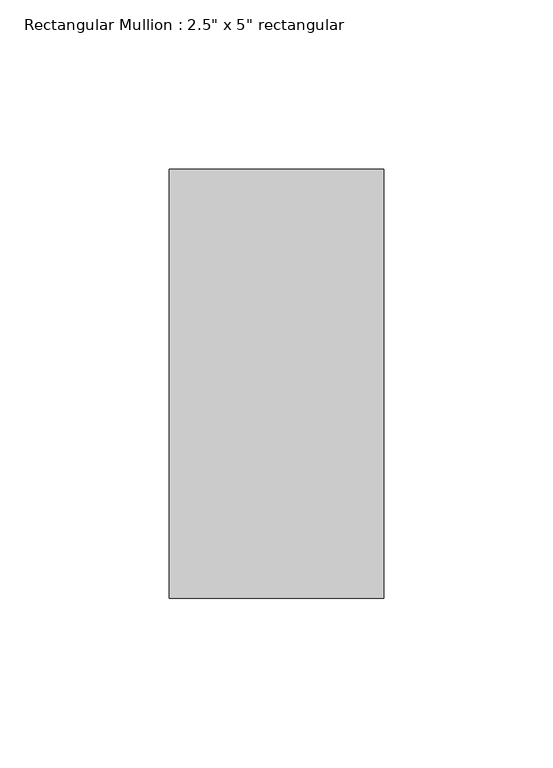
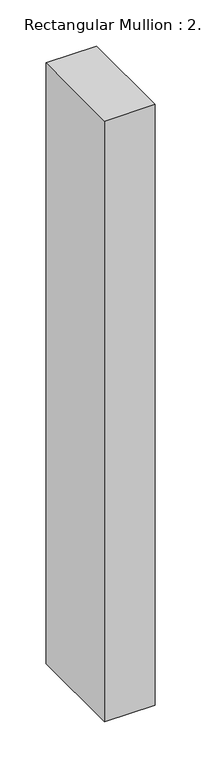
"""IFC4 building model written with IfcOpenShell, lengths in millimetres: member geometry."""

from ifc_helpers import new_model, si_unit, frame, origin, place, context, project, spatial, polyline, outline, extrude, source, transform, mapped, element, save


def member_952a807c(model_context):
    return source(origin(), model_context, "Body", "SweptSolid", [
        extrude(outline(polyline([(31.75, 63.5), (31.75, -63.5), (-31.75, -63.5), (-31.75, 63.5), (31.75, 63.5)])), frame((0.0, 0.0, -795.8666667), z_axis=(0.0, 0.0, 1.0), x_axis=(1.0, 0.0, 0.0)), (0.0, 0.0, 1.0), 795.8666667),
    ])


if __name__ == "__main__":
    model = new_model("IFC4")
    model_context = context("Model", 3, world=origin())
    ifc_project = project(units=[si_unit("LENGTHUNIT", "METRE", prefix="MILLI")], contexts=[model_context])
    site = spatial("IfcSite", under=ifc_project)
    building = spatial("IfcBuilding", under=site)
    placement = place(None, origin())
    member_shape = member_952a807c(model_context)
    element("IfcMember", 1, ObjectType="Rectangular Mullion : 2.5\" x 5\" rectangular", at=placement, inside=building, context=model_context, shape_type="MappedRepresentation", body=[
        mapped(member_shape, transform((0.0, 0.0, 0.0), x_axis=(1.0, 0.0, 0.0), y_axis=(0.0, 1.0, 0.0), z_axis=(0.0, 0.0, 1.0))),
    ])
    save(model, "model.ifc")

# Revit data of these elements
# Type "Rectangular Mullion : 2.5\" x 5\" rectangular"
#   built-in parameter 1007304 = 0.416667 (stored number, unit not read)
#   built-in parameter 1007301 = 0.104167 (stored number, unit not read)
#   built-in parameter 1007300 = 0.104167 (stored number, unit not read)
# Element 1 (IfcMember, "Rectangular Mullion : 2.5\" x 5\" rectangular")
#   Materials on its faces: "Aluminum"
# Materials
#   "Aluminum": class "Metal", colour RGB 247 247 247, transparency 0, Description = "Aluminum 6061", Cost = 0
